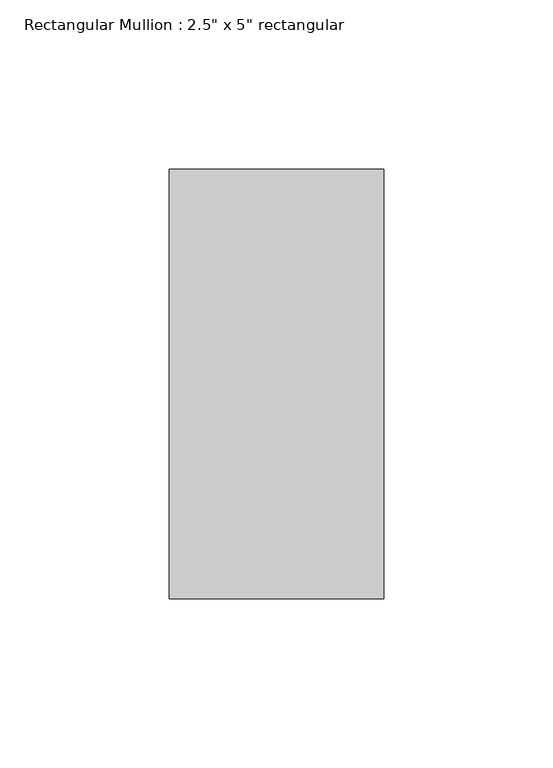
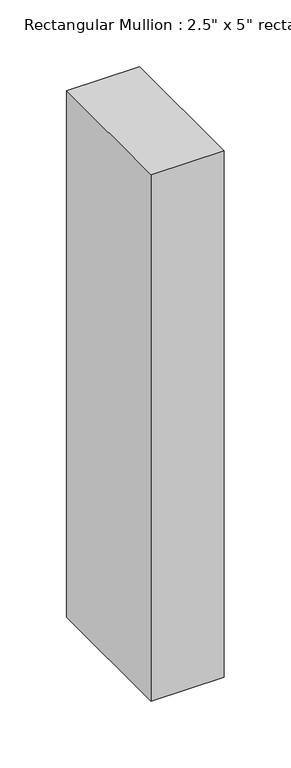
"""IFC4 building model written with IfcOpenShell, lengths in millimetres: member geometry."""

from ifc_helpers import new_model, si_unit, frame, origin, place, context, project, spatial, polyline, outline, extrude, source, transform, mapped, element, save


def member_86d06fe4(model_context):
    return source(origin(), model_context, "Body", "SweptSolid", [
        extrude(outline(polyline([(0.0, 63.5), (0.0, -63.5), (-63.5, -63.5), (-63.5, 63.5), (0.0, 63.5)])), frame((0.0, 0.0, -482.6), z_axis=(0.0, 0.0, 1.0), x_axis=(1.0, 0.0, 0.0)), (0.0, 0.0, 1.0), 482.6),
    ])


if __name__ == "__main__":
    model = new_model("IFC4")
    model_context = context("Model", 3, world=origin())
    ifc_project = project(units=[si_unit("LENGTHUNIT", "METRE", prefix="MILLI")], contexts=[model_context])
    site = spatial("IfcSite", under=ifc_project)
    building = spatial("IfcBuilding", under=site)
    placement = place(None, origin())
    member_shape = member_86d06fe4(model_context)
    element("IfcMember", 1, ObjectType="Rectangular Mullion : 2.5\" x 5\" rectangular", at=placement, inside=building, context=model_context, shape_type="MappedRepresentation", body=[
        mapped(member_shape, transform((0.0, 0.0, 0.0), x_axis=(1.0, 0.0, 0.0), y_axis=(0.0, 1.0, 0.0), z_axis=(0.0, 0.0, 1.0))),
    ])
    save(model, "model.ifc")

# Revit data of these elements
# Type "Rectangular Mullion : 2.5\" x 5\" rectangular"
#   built-in parameter 1007304 = 0.416667 (stored number, unit not read)
#   built-in parameter 1007301 = 0.104167 (stored number, unit not read)
#   built-in parameter 1007300 = 0.104167 (stored number, unit not read)
